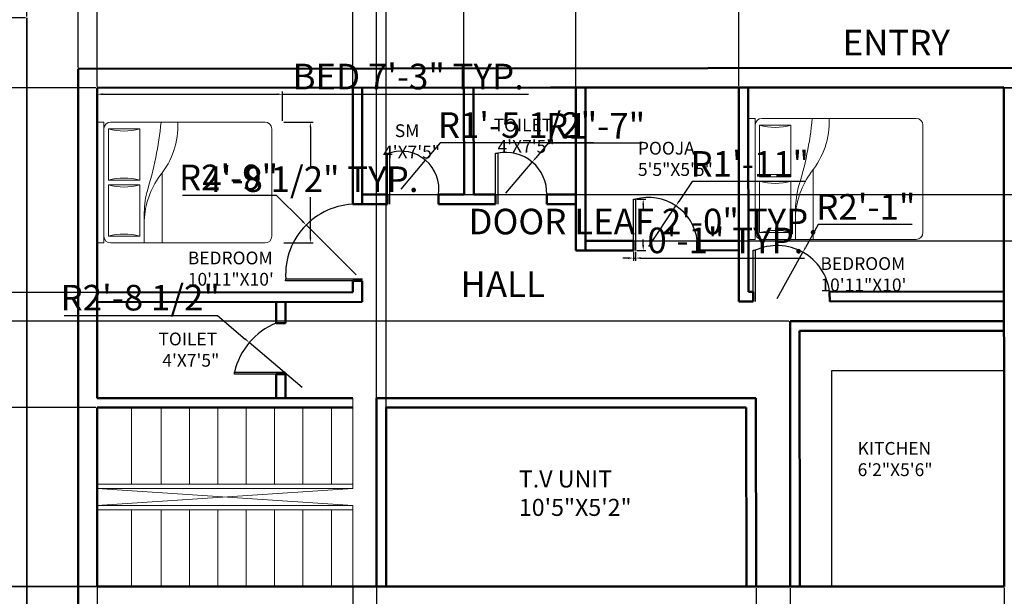
# Model space of a CAD drawing. Units: inches. Extents: x 5307 to 6359, y 4763 to 5474.
# Tile 3 of 5: x 5543 to 6006, y 4966 to 5237. Entities that reach past the tile are written whole.
import ezdxf
from ezdxf.enums import TextEntityAlignment as Align

# ---------------------------------------------------------------- set-up
doc = ezdxf.new("R2010")
doc.units = ezdxf.units.IN
for name, color, linetype, lineweight in [('A-ANNO-DIMS', 2, 'Continuous', 18), ('A-ANNO-TEXT', 7, 'Continuous', 18), ('A-AREA-IDEN', 7, 'Continuous', 18), ('A-DOOR', 4, 'Continuous', 25), ('A-FLOR-FIXT', 9, 'Continuous', 25), ('A-FLOR-STRS', 3, 'Continuous', 18), ('A-WALL', 7, 'Continuous', 50), ('C-PROP', 7, 'Continuous', 35), ('FUR', 42, 'Continuous', 18)]:
    doc.layers.add(name, color=color, linetype=linetype, lineweight=lineweight)
doc.styles.add('ATT', font='romans.shx')
doc.styles.get("Standard").update_dxf_attribs({"font": 'arial.ttf'})
doc.dimstyles.new('ISO-25', dxfattribs={"dimtxt": 12, "dimasz": 2.5, "dimexe": 1.25, "dimexo": 0.625, "dimtad": 1, "dimtih": 1, "dimtoh": 1, "dimlunit": 4, "dimtxsty": 'Standard', "dimcen": 2.5, "dimadec": 0, "dimazin": 0, "dimtfac": 1, "dimtmove": 0, "dimatfit": 3, "dimfxl": 1, "dimarcsym": 0})

# ---------------------------------------------------------------- blocks, each defined once
blk = doc.blocks.new('*D3')
at = {"layer": 'A-ANNO-DIMS', "color": 0, "lineweight": -2, "transparency": 16777216}
for p, q in [((5545.97, 5237.78), (5511.45, 5237.78)), ((5512.7, 5235.28), (5512.7, 5094.54)), ((5512.7, 4940.28), (5512.7, 5081.03)), ((5545.97, 4937.78), (5511.45, 4937.78))]:
    blk.add_line(p, q, dxfattribs=at)
at = {"layer": 'A-ANNO-DIMS', "color": 0, "transparency": 16777216}
for points in [[(5512.28, 5235.28), (5513.12, 5235.28), (5512.7, 5237.78)], [(5512.28, 4940.28), (5513.12, 4940.28), (5512.7, 4937.78)]]:
    blk.add_solid(points, dxfattribs=at)
at = {"layer": 'Defpoints', "color": 0, "transparency": 16777216}
for p in [(5546.59, 5237.78), (5512.7, 4937.78), (5546.59, 4937.78)]:
    blk.add_point(p, dxfattribs=at)
at = {"layer": 'A-ANNO-DIMS', "color": 0, "transparency": 16777216, "insert": (5512.7, 5087.78), "char_height": 12, "attachment_point": 5}
blk.add_mtext("25'", dxfattribs=at)
blk = doc.blocks.new('12PBED03')
at = {"color": 0, "linetype": 'ByBlock'}
for p, q in [((3, 54), (0, 54)), ((0, 0), (0, 54)), ((3, 0), (3, 54)), ((6, 54), (75, 54)), ((21, 41.758136), (21, 54)), ((29, 23), (29, 54)), ((19, 51), (5, 51)), ((5, 51), (5, 28)), ((19, 28), (19, 51)), ((78, 51), (78, 3)), ((5, 28), (19, 28)), ((5, 26), (5, 3)), ((19, 26), (5, 26)), ((19, 3), (19, 26)), ((3, 0), (0, 0)), ((5, 3), (19, 3)), ((75, 0), (6, 0))]:
    blk.add_line(p, q, dxfattribs=at)
for centre, radius, start, end in [((6, 51), 3, 90, 180), ((75, 51), 3, 0, 90), ((12, 75), 25, 253.739795, 286.260205), ((69.004289, 41.742518), 48.004291, 179.981359, 192.466744), ((57.725806, 45.629032), 36.761918, 182.539782, 216.040311), ((-120.191801, -13.95004), 149.36804, 5.357156, 17.666547), ((12, 4), 25, 73.739795, 106.260205), ((12, 50), 25, 253.739795, 286.260205), ((0.75, 1.5), 35.338541, 357.56726, 39.546081), ((6, 3), 3, 180, 270), ((12, -21), 25, 73.739795, 106.260205), ((75, 3), 3, 270, 0)]:
    blk.add_arc(centre, radius, start, end, dxfattribs=at)
at = {"color": 0, "linetype": 'ByBlock', "style": 'ATT'}
for tag, flags, p in [('ITEM', 3, (50, 33)), ('ROOM_NUMBER', 1, (50, 18.5))]:
    blk.add_attdef(tag, text='', height=6, dxfattribs=dict(at, flags=flags)).set_placement(p, align=Align.CENTER)
blk = doc.blocks.new('DOOR-LEAF-24IN')
for p, q in [((0, 0), (0, 24)), ((0, 24), (1, 24)), ((1, 24), (1, 0))]:
    blk.add_line(p, q)
blk = doc.blocks.new('*D8')
at = {"layer": 'A-ANNO-DIMS', "color": 0, "lineweight": -2, "transparency": 16777216}
for p, q in [((5833.01, 5152.56), (5837.24, 5152.56)), ((5835.99, 5150.06), (5835.99, 5147.39)), ((5835.99, 5131.06), (5835.99, 5133.73)), ((5833.01, 5128.56), (5837.24, 5128.56))]:
    blk.add_line(p, q, dxfattribs=at)
at = {"layer": 'A-ANNO-DIMS', "color": 0, "transparency": 16777216}
for points in [[(5835.57, 5150.06), (5836.4, 5150.06), (5835.99, 5152.56)], [(5835.57, 5131.06), (5836.4, 5131.06), (5835.99, 5128.56)]]:
    blk.add_solid(points, dxfattribs=at)
at = {"layer": 'Defpoints', "color": 0, "transparency": 16777216}
for p in [(5832.39, 5152.56), (5835.99, 5152.56), (5832.39, 5128.56)]:
    blk.add_point(p, dxfattribs=at)
at = {"layer": 'A-ANNO-DIMS', "color": 0, "transparency": 16777216, "insert": (5835.99, 5140.56), "char_height": 12, "attachment_point": 5}
blk.add_mtext('DOOR LEAF 2\'-0" TYP.', dxfattribs=at)
blk = doc.blocks.new('*D9')
at = {"layer": 'A-ANNO-DIMS', "color": 0, "lineweight": -2, "transparency": 16777216}
for p, q in [((5831.39, 5127.94), (5831.39, 5123.71)), ((5832.39, 5127.94), (5832.39, 5123.71)), ((5828.89, 5124.96), (5826.39, 5124.96)), ((5831.39, 5124.96), (5832.39, 5124.96)), ((5834.89, 5124.96), (5911.78, 5124.96))]:
    blk.add_line(p, q, dxfattribs=at)
at = {"layer": 'A-ANNO-DIMS', "color": 0, "transparency": 16777216}
for points in [[(5828.89, 5125.38), (5828.89, 5124.54), (5831.39, 5124.96)], [(5834.89, 5125.38), (5834.89, 5124.54), (5832.39, 5124.96)]]:
    blk.add_solid(points, dxfattribs=at)
at = {"layer": 'Defpoints', "color": 0, "transparency": 16777216}
for p in [(5831.39, 5128.56), (5832.39, 5128.56), (5832.39, 5124.96)]:
    blk.add_point(p, dxfattribs=at)
at = {"layer": 'A-ANNO-DIMS', "color": 0, "transparency": 16777216, "insert": (5874.59, 5131.71), "char_height": 12, "attachment_point": 5}
blk.add_mtext('0\'-1" TYP.', dxfattribs=at)
blk = doc.blocks.new('*D10')
at = {"layer": 'A-ANNO-DIMS', "color": 0, "lineweight": -2, "transparency": 16777216}
for p, q in [((5579.59, 5189.42), (5579.59, 5203.11)), ((5582.09, 5201.86), (5664.17, 5201.86)), ((5666.67, 5189.42), (5666.67, 5203.11)), ((5666.67, 5201.86), (5782.16, 5201.86))]:
    blk.add_line(p, q, dxfattribs=at)
at = {"layer": 'A-ANNO-DIMS', "color": 0, "transparency": 16777216}
for points in [[(5582.09, 5202.27), (5582.09, 5201.44), (5579.59, 5201.86)], [(5664.17, 5202.27), (5664.17, 5201.44), (5666.67, 5201.86)]]:
    blk.add_solid(points, dxfattribs=at)
at = {"layer": 'Defpoints', "color": 0, "transparency": 16777216}
for p in [(5666.67, 5201.86), (5579.59, 5188.79), (5666.67, 5188.79)]:
    blk.add_point(p, dxfattribs=at)
at = {"layer": 'A-ANNO-DIMS', "color": 0, "transparency": 16777216, "insert": (5725.66, 5208.61), "char_height": 12, "attachment_point": 5}
blk.add_mtext('BED 7\'-3" TYP.', dxfattribs=at)
blk = doc.blocks.new('*D11')
at = {"layer": 'A-ANNO-DIMS', "color": 0, "lineweight": -2, "transparency": 16777216}
for p, q in [((5667.29, 5188.79), (5680.98, 5188.79)), ((5679.73, 5186.29), (5679.73, 5167.25)), ((5679.73, 5134.55), (5679.73, 5153.59)), ((5667.29, 5132.05), (5680.98, 5132.05))]:
    blk.add_line(p, q, dxfattribs=at)
at = {"layer": 'A-ANNO-DIMS', "color": 0, "transparency": 16777216}
for points in [[(5679.31, 5186.29), (5680.14, 5186.29), (5679.73, 5188.79)], [(5679.31, 5134.55), (5680.14, 5134.55), (5679.73, 5132.05)]]:
    blk.add_solid(points, dxfattribs=at)
at = {"layer": 'Defpoints', "color": 0, "transparency": 16777216}
for p in [(5666.67, 5188.79), (5666.67, 5132.05), (5679.73, 5132.05)]:
    blk.add_point(p, dxfattribs=at)
at = {"layer": 'A-ANNO-DIMS', "color": 0, "transparency": 16777216, "insert": (5679.73, 5160.42), "char_height": 12, "attachment_point": 5}
blk.add_mtext('4\'-8 1/2" TYP.', dxfattribs=at)
blk = doc.blocks.new('*D13')
at = {"layer": 'A-ANNO-DIMS', "color": 0, "lineweight": -2, "transparency": 16777216}
for p, q in [((6038.88, 5405.78), (6325.25, 5405.78)), ((6324, 5403.28), (6324, 5118.54)), ((6324, 4820.28), (6324, 5105.03)), ((5547.22, 4817.78), (6325.25, 4817.78))]:
    blk.add_line(p, q, dxfattribs=at)
at = {"layer": 'A-ANNO-DIMS', "color": 0, "transparency": 16777216}
for points in [[(6323.58, 5403.28), (6324.41, 5403.28), (6324, 5405.78)], [(6323.58, 4820.28), (6324.41, 4820.28), (6324, 4817.78)]]:
    blk.add_solid(points, dxfattribs=at)
at = {"layer": 'Defpoints', "color": 0, "transparency": 16777216}
for p in [(6038.25, 5405.78), (6324, 5405.78), (5546.59, 4817.78)]:
    blk.add_point(p, dxfattribs=at)
at = {"layer": 'A-ANNO-DIMS', "color": 0, "transparency": 16777216, "insert": (6324, 5111.78), "char_height": 12, "attachment_point": 5}
blk.add_mtext('49\'-0"', dxfattribs=at)
blk = doc.blocks.new('*D14')
at = {"layer": 'A-ANNO-DIMS', "color": 0, "lineweight": -2, "transparency": 16777216}
for p, q in [((5546.59, 5238.41), (5546.59, 5450.78)), ((5549.09, 5449.53), (5568.09, 5449.53)), ((5570.59, 5214.43), (5570.59, 5450.78)), ((5570.59, 5449.53), (5606.45, 5449.53))]:
    blk.add_line(p, q, dxfattribs=at)
at = {"layer": 'A-ANNO-DIMS', "color": 0, "transparency": 16777216}
for points in [[(5549.09, 5449.95), (5549.09, 5449.12), (5546.59, 5449.53)], [(5568.09, 5449.95), (5568.09, 5449.12), (5570.59, 5449.53)]]:
    blk.add_solid(points, dxfattribs=at)
at = {"layer": 'Defpoints', "color": 0, "transparency": 16777216}
for p in [(5570.59, 5449.53), (5546.59, 5237.78), (5570.59, 5213.81)]:
    blk.add_point(p, dxfattribs=at)
at = {"layer": 'A-ANNO-DIMS', "color": 0, "transparency": 16777216, "insert": (5589.77, 5456.29), "char_height": 12, "attachment_point": 5}
blk.add_mtext('2\'-0"', dxfattribs=at)
blk = doc.blocks.new('*D19')
at = {"layer": 'A-ANNO-DIMS', "color": 0, "lineweight": -2, "transparency": 16777216}
for p, q in [((5570.59, 5214.43), (5570.59, 5450.78)), ((5573.09, 5449.53), (5577.09, 5449.53)), ((5579.59, 5205.44), (5579.59, 5450.78)), ((5579.59, 5449.53), (5615.24, 5449.53))]:
    blk.add_line(p, q, dxfattribs=at)
at = {"layer": 'A-ANNO-DIMS', "color": 0, "transparency": 16777216}
for points in [[(5573.09, 5449.95), (5573.09, 5449.12), (5570.59, 5449.53)], [(5577.09, 5449.95), (5577.09, 5449.12), (5579.59, 5449.53)]]:
    blk.add_solid(points, dxfattribs=at)
at = {"layer": 'Defpoints', "color": 0, "transparency": 16777216}
for p in [(5579.59, 5449.53), (5570.59, 5213.81), (5579.59, 5204.82)]:
    blk.add_point(p, dxfattribs=at)
at = {"layer": 'A-ANNO-DIMS', "color": 0, "transparency": 16777216, "insert": (5598.67, 5456.29), "char_height": 12, "attachment_point": 5}
blk.add_mtext('0\'-9"', dxfattribs=at)
blk = doc.blocks.new('*D20')
at = {"layer": 'A-ANNO-DIMS', "color": 0, "lineweight": -2, "transparency": 16777216}
for p, q in [((5579.59, 5205.44), (5579.59, 5450.78)), ((5582.09, 5449.53), (5697.09, 5449.53)), ((5699.59, 5205.56), (5699.59, 5450.78))]:
    blk.add_line(p, q, dxfattribs=at)
at = {"layer": 'A-ANNO-DIMS', "color": 0, "transparency": 16777216}
for points in [[(5582.09, 5449.95), (5582.09, 5449.12), (5579.59, 5449.53)], [(5697.09, 5449.95), (5697.09, 5449.12), (5699.59, 5449.53)]]:
    blk.add_solid(points, dxfattribs=at)
at = {"layer": 'Defpoints', "color": 0, "transparency": 16777216}
for p in [(5699.59, 5449.53), (5579.59, 5204.82), (5699.59, 5204.93)]:
    blk.add_point(p, dxfattribs=at)
at = {"layer": 'A-ANNO-DIMS', "color": 0, "transparency": 16777216, "insert": (5639.59, 5456.29), "char_height": 12, "attachment_point": 5}
blk.add_mtext('10\'-0"', dxfattribs=at)
blk = doc.blocks.new('*D21')
at = {"layer": 'A-ANNO-DIMS', "color": 0, "lineweight": -2, "transparency": 16777216}
for p, q in [((5699.59, 5205.56), (5699.59, 5450.78)), ((5702.09, 5449.53), (5749.33, 5449.53)), ((5751.83, 5205.61), (5751.83, 5450.78))]:
    blk.add_line(p, q, dxfattribs=at)
at = {"layer": 'A-ANNO-DIMS', "color": 0, "transparency": 16777216}
for points in [[(5702.09, 5449.95), (5702.09, 5449.12), (5699.59, 5449.53)], [(5749.33, 5449.95), (5749.33, 5449.12), (5751.83, 5449.53)]]:
    blk.add_solid(points, dxfattribs=at)
at = {"layer": 'Defpoints', "color": 0, "transparency": 16777216}
for p in [(5751.83, 5449.53), (5699.59, 5204.93), (5751.83, 5204.98)]:
    blk.add_point(p, dxfattribs=at)
at = {"layer": 'A-ANNO-DIMS', "color": 0, "transparency": 16777216, "insert": (5725.71, 5456.16), "char_height": 12, "attachment_point": 5}
blk.add_mtext('4\'-4"', dxfattribs=at)
blk = doc.blocks.new('*D22')
at = {"layer": 'A-ANNO-DIMS', "color": 0, "lineweight": -2, "transparency": 16777216}
for p, q in [((5751.83, 5205.61), (5751.83, 5450.78)), ((5754.33, 5449.53), (5801.83, 5449.53)), ((5804.33, 5205.66), (5804.33, 5450.78)), ((5804.33, 5449.53), (5868.43, 5449.53))]:
    blk.add_line(p, q, dxfattribs=at)
at = {"layer": 'A-ANNO-DIMS', "color": 0, "transparency": 16777216}
for points in [[(5754.33, 5449.95), (5754.33, 5449.12), (5751.83, 5449.53)], [(5801.83, 5449.95), (5801.83, 5449.12), (5804.33, 5449.53)]]:
    blk.add_solid(points, dxfattribs=at)
at = {"layer": 'Defpoints', "color": 0, "transparency": 16777216}
for p in [(5804.33, 5449.53), (5751.83, 5204.98), (5804.33, 5205.03)]:
    blk.add_point(p, dxfattribs=at)
at = {"layer": 'A-ANNO-DIMS', "color": 0, "transparency": 16777216, "insert": (5837.63, 5456.36), "char_height": 12, "attachment_point": 5}
blk.add_mtext('4\'-4 1/2"', dxfattribs=at)
blk = doc.blocks.new('*D23')
at = {"layer": 'A-ANNO-DIMS', "color": 0, "lineweight": -2, "transparency": 16777216}
for p, q in [((5804.33, 5205.66), (5804.33, 5450.78)), ((5806.83, 5449.53), (5878.33, 5449.53)), ((5880.83, 5205.73), (5880.83, 5450.78))]:
    blk.add_line(p, q, dxfattribs=at)
at = {"layer": 'A-ANNO-DIMS', "color": 0, "transparency": 16777216}
for points in [[(5806.83, 5449.95), (5806.83, 5449.12), (5804.33, 5449.53)], [(5878.33, 5449.95), (5878.33, 5449.12), (5880.83, 5449.53)]]:
    blk.add_solid(points, dxfattribs=at)
at = {"layer": 'Defpoints', "color": 0, "transparency": 16777216}
for p in [(5880.83, 5449.53), (5804.33, 5205.03), (5880.83, 5205.11)]:
    blk.add_point(p, dxfattribs=at)
at = {"layer": 'A-ANNO-DIMS', "color": 0, "transparency": 16777216, "insert": (5842.58, 5456.36), "char_height": 12, "attachment_point": 5}
blk.add_mtext('6\'-4 1/2"', dxfattribs=at)
blk = doc.blocks.new('*D24')
at = {"layer": 'A-ANNO-DIMS', "color": 0, "lineweight": -2, "transparency": 16777216}
for p, q in [((5579.59, 4970.16), (5579.59, 4772.78)), ((5699.59, 4970.16), (5699.59, 4772.78)), ((5582.09, 4774.03), (5697.09, 4774.03))]:
    blk.add_line(p, q, dxfattribs=at)
at = {"layer": 'A-ANNO-DIMS', "color": 0, "transparency": 16777216}
for points in [[(5582.09, 4774.45), (5582.09, 4773.62), (5579.59, 4774.03)], [(5697.09, 4774.45), (5697.09, 4773.62), (5699.59, 4774.03)]]:
    blk.add_solid(points, dxfattribs=at)
at = {"layer": 'Defpoints', "color": 0, "transparency": 16777216}
for p in [(5579.59, 4970.78), (5699.59, 4970.78), (5699.59, 4774.03)]:
    blk.add_point(p, dxfattribs=at)
at = {"layer": 'A-ANNO-DIMS', "color": 0, "transparency": 16777216, "insert": (5639.59, 4780.79), "char_height": 12, "attachment_point": 5}
blk.add_mtext('10\'-0"', dxfattribs=at)
blk = doc.blocks.new('*D25')
at = {"layer": 'A-ANNO-DIMS', "color": 0, "lineweight": -2, "transparency": 16777216}
for p, q in [((5710.76, 4970.16), (5710.76, 4772.78)), ((5889, 4970.05), (5889, 4772.78)), ((5713.26, 4774.03), (5886.5, 4774.03))]:
    blk.add_line(p, q, dxfattribs=at)
at = {"layer": 'A-ANNO-DIMS', "color": 0, "transparency": 16777216}
for points in [[(5713.26, 4774.45), (5713.26, 4773.62), (5710.76, 4774.03)], [(5886.5, 4774.45), (5886.5, 4773.62), (5889, 4774.03)]]:
    blk.add_solid(points, dxfattribs=at)
at = {"layer": 'Defpoints', "color": 0, "transparency": 16777216}
for p in [(5710.76, 4970.78), (5889, 4970.67), (5889, 4774.03)]:
    blk.add_point(p, dxfattribs=at)
at = {"layer": 'A-ANNO-DIMS', "color": 0, "transparency": 16777216, "insert": (5799.88, 4780.79), "char_height": 12, "attachment_point": 5}
blk.add_mtext('14\'-10"', dxfattribs=at)
blk = doc.blocks.new('*D26')
at = {"layer": 'A-ANNO-DIMS', "color": 0, "lineweight": -2, "transparency": 16777216}
for p, q in [((5905.06, 4970.06), (5905.06, 4772.78)), ((6005.56, 4970.16), (6005.56, 4772.78)), ((5907.56, 4774.03), (6003.06, 4774.03))]:
    blk.add_line(p, q, dxfattribs=at)
at = {"layer": 'A-ANNO-DIMS', "color": 0, "transparency": 16777216}
for points in [[(5907.56, 4774.45), (5907.56, 4773.62), (5905.06, 4774.03)], [(6003.06, 4774.45), (6003.06, 4773.62), (6005.56, 4774.03)]]:
    blk.add_solid(points, dxfattribs=at)
at = {"layer": 'Defpoints', "color": 0, "transparency": 16777216}
for p in [(5905.06, 4970.69), (6005.56, 4970.78), (6005.56, 4774.03)]:
    blk.add_point(p, dxfattribs=at)
at = {"layer": 'A-ANNO-DIMS', "color": 0, "transparency": 16777216, "insert": (5955.31, 4780.86), "char_height": 12, "attachment_point": 5}
blk.add_mtext('8\'-4 1/2"', dxfattribs=at)
blk = doc.blocks.new('*D27')
at = {"layer": 'A-ANNO-DIMS', "color": 0, "lineweight": -2, "transparency": 16777216}
for p, q in [((5578.97, 5054.78), (5381.59, 5054.78)), ((5382.84, 5052.28), (5382.84, 5019.54)), ((5382.84, 4973.28), (5382.84, 5006.03)), ((5578.97, 4970.78), (5381.59, 4970.78))]:
    blk.add_line(p, q, dxfattribs=at)
at = {"layer": 'A-ANNO-DIMS', "color": 0, "transparency": 16777216}
for points in [[(5382.43, 5052.28), (5383.26, 5052.28), (5382.84, 5054.78)], [(5382.43, 4973.28), (5383.26, 4973.28), (5382.84, 4970.78)]]:
    blk.add_solid(points, dxfattribs=at)
at = {"layer": 'Defpoints', "color": 0, "transparency": 16777216}
for p in [(5382.84, 5054.78), (5579.59, 5054.78), (5579.59, 4970.78)]:
    blk.add_point(p, dxfattribs=at)
at = {"layer": 'A-ANNO-DIMS', "color": 0, "transparency": 16777216, "insert": (5382.84, 5012.78), "char_height": 12, "attachment_point": 5}
blk.add_mtext('7\'-0"', dxfattribs=at)
blk = doc.blocks.new('*D28')
at = {"layer": 'A-ANNO-DIMS', "color": 0, "lineweight": -2, "transparency": 16777216}
for p, q in [((5578.97, 5204.82), (5381.59, 5204.82)), ((5382.84, 5202.32), (5382.84, 5163.57)), ((5382.84, 5111.32), (5382.84, 5150.06)), ((5578.97, 5108.82), (5381.59, 5108.82))]:
    blk.add_line(p, q, dxfattribs=at)
at = {"layer": 'A-ANNO-DIMS', "color": 0, "transparency": 16777216}
for points in [[(5382.43, 5202.32), (5383.26, 5202.32), (5382.84, 5204.82)], [(5382.43, 5111.32), (5383.26, 5111.32), (5382.84, 5108.82)]]:
    blk.add_solid(points, dxfattribs=at)
at = {"layer": 'Defpoints', "color": 0, "transparency": 16777216}
for p in [(5382.84, 5204.82), (5579.59, 5204.82), (5579.59, 5108.82)]:
    blk.add_point(p, dxfattribs=at)
at = {"layer": 'A-ANNO-DIMS', "color": 0, "transparency": 16777216, "insert": (5382.84, 5156.82), "char_height": 12, "attachment_point": 5}
blk.add_mtext('8\'-0"', dxfattribs=at)
blk = doc.blocks.new('*D29')
at = {"layer": 'A-ANNO-DIMS', "color": 0, "lineweight": -2, "transparency": 16777216}
for p, q in [((5904.31, 5095.28), (5381.59, 5095.28)), ((5382.84, 5092.78), (5382.84, 5039.81)), ((5382.84, 4973.19), (5382.84, 5026.16)), ((5904.44, 4970.69), (5381.59, 4970.69))]:
    blk.add_line(p, q, dxfattribs=at)
at = {"layer": 'A-ANNO-DIMS', "color": 0, "transparency": 16777216}
for points in [[(5382.43, 5092.78), (5383.26, 5092.78), (5382.84, 5095.28)], [(5382.43, 4973.19), (5383.26, 4973.19), (5382.84, 4970.69)]]:
    blk.add_solid(points, dxfattribs=at)
at = {"layer": 'Defpoints', "color": 0, "transparency": 16777216}
for p in [(5382.84, 5095.28), (5904.94, 5095.28), (5905.06, 4970.69)]:
    blk.add_point(p, dxfattribs=at)
at = {"layer": 'A-ANNO-DIMS', "color": 0, "transparency": 16777216, "insert": (5382.84, 5032.99), "char_height": 12, "attachment_point": 5}
blk.add_mtext('10\'-4 1/2"', dxfattribs=at)
blk = doc.blocks.new('*D30')
at = {"layer": 'A-ANNO-DIMS', "color": 0, "lineweight": -2, "transparency": 16777216}
for p, q in [((5708.26, 5449.53), (5705.76, 5449.53)), ((5710.76, 4971.41), (5710.76, 5450.78)), ((5710.76, 5449.53), (5715.26, 5449.53)), ((5715.26, 4971.41), (5715.26, 5450.78)), ((5717.76, 5449.53), (5781.37, 5449.53))]:
    blk.add_line(p, q, dxfattribs=at)
at = {"layer": 'A-ANNO-DIMS', "color": 0, "transparency": 16777216}
for points in [[(5708.26, 5449.95), (5708.26, 5449.12), (5710.76, 5449.53)], [(5717.76, 5449.95), (5717.76, 5449.12), (5715.26, 5449.53)]]:
    blk.add_solid(points, dxfattribs=at)
at = {"layer": 'Defpoints', "color": 0, "transparency": 16777216}
for p in [(5715.26, 5449.53), (5710.76, 4970.78), (5715.26, 4970.78)]:
    blk.add_point(p, dxfattribs=at)
at = {"layer": 'A-ANNO-DIMS', "color": 0, "transparency": 16777216, "insert": (5750.81, 5456.36), "char_height": 12, "attachment_point": 5}
blk.add_mtext('0\'-4 1/2"', dxfattribs=at)
blk = doc.blocks.new('*D31')
at = {"layer": 'A-ANNO-DIMS', "color": 0, "lineweight": -2, "transparency": 16777216}
for p, q in [((5704.72, 5204.94), (6325.25, 5204.94)), ((6324, 5202.44), (6324, 5186.48)), ((6324, 5157.23), (6324, 5173.19)), ((5704.72, 5154.73), (6325.25, 5154.73))]:
    blk.add_line(p, q, dxfattribs=at)
at = {"layer": 'A-ANNO-DIMS', "color": 0, "transparency": 16777216}
for points in [[(6323.58, 5202.44), (6324.41, 5202.44), (6324, 5204.94)], [(6323.58, 5157.23), (6324.41, 5157.23), (6324, 5154.73)]]:
    blk.add_solid(points, dxfattribs=at)
at = {"layer": 'Defpoints', "color": 0, "transparency": 16777216}
for p in [(5704.09, 5204.94), (6324, 5204.94), (5704.09, 5154.73)]:
    blk.add_point(p, dxfattribs=at)
at = {"layer": 'A-ANNO-DIMS', "color": 0, "transparency": 16777216, "insert": (6324, 5179.83), "char_height": 12, "attachment_point": 5}
blk.add_mtext('4\'-2"', dxfattribs=at)
blk = doc.blocks.new('*D32')
at = {"layer": 'A-ANNO-DIMS', "color": 0, "lineweight": -2, "transparency": 16777216}
for p, q in [((5809.46, 5205.04), (6325.25, 5205.04)), ((6324, 5202.54), (6324, 5175.79)), ((6324, 5135.54), (6324, 5162.29)), ((5809.53, 5133.04), (6325.25, 5133.04))]:
    blk.add_line(p, q, dxfattribs=at)
at = {"layer": 'A-ANNO-DIMS', "color": 0, "transparency": 16777216}
for points in [[(6323.58, 5202.54), (6324.41, 5202.54), (6324, 5205.04)], [(6323.58, 5135.54), (6324.41, 5135.54), (6324, 5133.04)]]:
    blk.add_solid(points, dxfattribs=at)
at = {"layer": 'Defpoints', "color": 0, "transparency": 16777216}
for p in [(5808.83, 5205.04), (6324, 5205.04), (5808.9, 5133.04)]:
    blk.add_point(p, dxfattribs=at)
at = {"layer": 'A-ANNO-DIMS', "color": 0, "transparency": 16777216, "insert": (6324, 5169.04), "char_height": 12, "attachment_point": 5}
blk.add_mtext('6\'-0"', dxfattribs=at)
blk = doc.blocks.new('*D35')
at = {"layer": 'A-ANNO-DIMS', "color": 0, "lineweight": -2, "transparency": 16777216}
for p, q in [((5619.59, 5154.53), (5663.6, 5154.53)), ((5663.6, 5154.53), (5675.95, 5142.25)), ((5701.26, 5117.08), (5677.72, 5140.49))]:
    blk.add_line(p, q, dxfattribs=at)
at = {"layer": 'A-ANNO-DIMS', "color": 0, "transparency": 16777216}
blk.add_solid([(5676.24, 5142.55), (5675.65, 5141.95), (5677.72, 5140.49)], dxfattribs=at)
at = {"layer": 'Defpoints', "color": 0, "transparency": 16777216}
for p in [(5677.72, 5140.49), (5701.26, 5117.08)]:
    blk.add_point(p, dxfattribs=at)
at = {"layer": 'A-ANNO-DIMS', "color": 0, "transparency": 16777216, "insert": (5641.28, 5161.28), "char_height": 12, "attachment_point": 5}
blk.add_mtext('R2\'-9"', dxfattribs=at)
blk = doc.blocks.new('*D36')
at = {"layer": 'A-ANNO-DIMS', "color": 0, "lineweight": -2, "transparency": 16777216}
for p, q in [((5564.14, 5098), (5636.11, 5098)), ((5636.11, 5098), (5649.11, 5086.98)), ((5675.87, 5064.29), (5651.02, 5085.36))]:
    blk.add_line(p, q, dxfattribs=at)
at = {"layer": 'A-ANNO-DIMS', "color": 0, "transparency": 16777216}
blk.add_solid([(5649.38, 5087.29), (5648.85, 5086.66), (5651.02, 5085.36)], dxfattribs=at)
at = {"layer": 'Defpoints', "color": 0, "transparency": 16777216}
for p in [(5651.02, 5085.36), (5675.87, 5064.29)]:
    blk.add_point(p, dxfattribs=at)
at = {"layer": 'A-ANNO-DIMS', "color": 0, "transparency": 16777216, "insert": (5599.81, 5104.83), "char_height": 12, "attachment_point": 5}
blk.add_mtext('R2\'-8 1/2"', dxfattribs=at)
blk = doc.blocks.new('*D37')
at = {"layer": 'A-ANNO-DIMS', "color": 0, "lineweight": -2, "transparency": 16777216}
for p, q in [((5918.23, 5140.77), (5912.18, 5129.89)), ((5962.24, 5140.77), (5918.23, 5140.77)), ((5898.85, 5105.95), (5910.97, 5127.71))]:
    blk.add_line(p, q, dxfattribs=at)
at = {"layer": 'A-ANNO-DIMS', "color": 0, "transparency": 16777216}
blk.add_solid([(5911.82, 5130.1), (5912.54, 5129.69), (5910.97, 5127.71)], dxfattribs=at)
at = {"layer": 'Defpoints', "color": 0, "transparency": 16777216}
for p in [(5910.97, 5127.71), (5898.85, 5105.95)]:
    blk.add_point(p, dxfattribs=at)
at = {"layer": 'A-ANNO-DIMS', "color": 0, "transparency": 16777216, "insert": (5940.55, 5147.42), "char_height": 12, "attachment_point": 5}
blk.add_mtext('R2\'-1"', dxfattribs=at)
blk = doc.blocks.new('*D38')
at = {"layer": 'A-ANNO-DIMS', "color": 0, "lineweight": -2, "transparency": 16777216}
for p, q in [((5859.06, 5160.95), (5852.76, 5151.58)), ((5912.39, 5160.95), (5859.06, 5160.95)), ((5838.56, 5130.42), (5851.37, 5149.5))]:
    blk.add_line(p, q, dxfattribs=at)
at = {"layer": 'A-ANNO-DIMS', "color": 0, "transparency": 16777216}
blk.add_solid([(5852.42, 5151.81), (5853.11, 5151.34), (5851.37, 5149.5)], dxfattribs=at)
at = {"layer": 'Defpoints', "color": 0, "transparency": 16777216}
for p in [(5851.37, 5149.5), (5838.56, 5130.42)]:
    blk.add_point(p, dxfattribs=at)
at = {"layer": 'A-ANNO-DIMS', "color": 0, "transparency": 16777216, "insert": (5886.03, 5167.6), "char_height": 12, "attachment_point": 5}
blk.add_mtext('R1\'-11"', dxfattribs=at)
blk = doc.blocks.new('*D39')
at = {"layer": 'A-ANNO-DIMS', "color": 0, "lineweight": -2, "transparency": 16777216}
for p, q in [((5791.33, 5178.82), (5785.53, 5171.95)), ((5835.34, 5178.82), (5791.33, 5178.82)), ((5771.55, 5155.4), (5783.91, 5170.04))]:
    blk.add_line(p, q, dxfattribs=at)
at = {"layer": 'A-ANNO-DIMS', "color": 0, "transparency": 16777216}
blk.add_solid([(5785.21, 5172.21), (5785.84, 5171.68), (5783.91, 5170.04)], dxfattribs=at)
at = {"layer": 'Defpoints', "color": 0, "transparency": 16777216}
for p in [(5783.91, 5170.04), (5771.55, 5155.4)]:
    blk.add_point(p, dxfattribs=at)
at = {"layer": 'A-ANNO-DIMS', "color": 0, "transparency": 16777216, "insert": (5813.64, 5185.46), "char_height": 12, "attachment_point": 5}
blk.add_mtext('R1\'-7"', dxfattribs=at)
blk = doc.blocks.new('*D40')
at = {"layer": 'A-ANNO-DIMS', "color": 0, "lineweight": -2, "transparency": 16777216}
for p, q in [((5740.66, 5179), (5735.4, 5172.79)), ((5812.63, 5179), (5740.66, 5179)), ((5722.31, 5157.36), (5733.78, 5170.89))]:
    blk.add_line(p, q, dxfattribs=at)
at = {"layer": 'A-ANNO-DIMS', "color": 0, "transparency": 16777216}
blk.add_solid([(5735.08, 5173.06), (5735.72, 5172.52), (5733.78, 5170.89)], dxfattribs=at)
at = {"layer": 'Defpoints', "color": 0, "transparency": 16777216}
for p in [(5733.78, 5170.89), (5722.31, 5157.36)]:
    blk.add_point(p, dxfattribs=at)
at = {"layer": 'A-ANNO-DIMS', "color": 0, "transparency": 16777216, "insert": (5776.96, 5185.83), "char_height": 12, "attachment_point": 5}
blk.add_mtext('R1\'-5 1/2"', dxfattribs=at)

msp = doc.modelspace()

# ---------------------------------------------------------------- linework, layer by layer
at = {"layer": 'A-DOOR'}
for p, q in [((5887.558, 5128.615), (5888.558, 5128.624)), ((5887.558, 5104.615), (5887.558, 5128.615)), ((5888.558, 5128.624), (5888.558, 5104.624)), ((5668.092, 5114.233), (5668.113, 5115.233)), ((5704.092, 5114.233), (5668.092, 5114.233)), ((5668.113, 5115.233), (5704.113, 5115.258))]:
    msp.add_line(p, q, dxfattribs=at)
for centre, radius, start, end in [((5722.312, 5157.356), 17.737, 351.4949, 107.9208), ((5771.552, 5155.403), 19.154, 358.00742, 101.6178), ((5838.558, 5130.423), 22.981, 6.66301, 105.57332), ((5701.257, 5117.08), 33.195, 87.1266, 183.18977), ((5898.855, 5105.946), 24.906, 7.39056, 114.41916), ((5675.874, 5064.289), 32.582, 112.14418, 167.27152)]:
    msp.add_arc(centre, radius, start, end, dxfattribs=at)
at = {"layer": 'A-FLOR-FIXT'}
for p, q in [((6005.462, 5071.994), (5924.438, 5071.994)), ((5924.438, 5071.994), (5924.438, 4970.784)), ((6005.462, 5071.994), (6005.462, 5071.994))]:
    msp.add_line(p, q, dxfattribs=at)
at = {"layer": 'A-FLOR-STRS'}
for p, q in [((5699.592, 5059.284), (5699.592, 5016.784)), ((5595.715, 5054.784), (5595.715, 5018.784)), ((5609.561, 5054.784), (5609.561, 5018.784)), ((5622.894, 5054.784), (5622.894, 5018.784)), ((5636.227, 5054.784), (5636.227, 5018.784)), ((5649.561, 5054.784), (5649.561, 5018.784)), ((5662.894, 5054.784), (5662.894, 5018.784)), ((5676.227, 5054.784), (5676.227, 5018.784)), ((5689.561, 5054.784), (5689.561, 5018.784)), ((5699.592, 5048.946), (5699.592, 5016.784)), ((5579.592, 5018.784), (5699.592, 5018.784)), ((5579.592, 5016.784), (5699.592, 5016.784)), ((5579.592, 5016.784), (5699.592, 5008.784)), ((5699.592, 5016.784), (5579.592, 5008.784)), ((5579.592, 5008.784), (5699.592, 5008.784)), ((5699.592, 5008.784), (5699.592, 4970.784)), ((5699.592, 5008.784), (5699.592, 4970.784)), ((5579.592, 5006.784), (5699.592, 5006.784)), ((5595.715, 5006.784), (5595.715, 4970.784)), ((5609.561, 5006.784), (5609.561, 4970.784)), ((5622.894, 5006.784), (5622.894, 4970.784)), ((5636.227, 5006.784), (5636.227, 4970.784)), ((5649.561, 5006.784), (5649.561, 4970.784)), ((5662.894, 5006.784), (5662.894, 4970.784)), ((5676.227, 5006.784), (5676.227, 4970.784)), ((5689.561, 5006.784), (5689.561, 4970.784))]:
    msp.add_line(p, q, dxfattribs=at)
at = {"layer": 'A-WALL'}
for p, q in [((5570.592, 5213.807), (6014.324, 5214.238)), ((5570.592, 5213.807), (5570.592, 4961.784)), ((5579.592, 5204.816), (6005.333, 5205.229)), ((5579.592, 5204.816), (5579.592, 5059.284)), ((5699.592, 5204.932), (5699.592, 5150.233)), ((5704.092, 5204.937), (5704.092, 5150.233)), ((5751.882, 5154.733), (5751.833, 5204.983)), ((5756.382, 5154.737), (5756.333, 5204.987)), ((5804.407, 5128.534), (5804.333, 5205.034)), ((5808.907, 5128.538), (5808.833, 5205.038)), ((5880.931, 5104.608), (5880.833, 5205.108)), ((5885.426, 5109.112), (5885.333, 5205.112)), ((6005.56, 4970.784), (6005.333, 5205.229)), ((5715.854, 5154.733), (5704.092, 5154.733)), ((5715.854, 5154.733), (5715.854, 5150.233)), ((5751.886, 5154.733), (5739.854, 5154.733)), ((5739.854, 5154.733), (5739.854, 5150.233)), ((5756.382, 5154.737), (5766.694, 5154.737)), ((5766.694, 5154.737), (5766.694, 5150.237)), ((5790.694, 5154.737), (5790.694, 5150.237)), ((5790.694, 5154.737), (5804.382, 5154.737)), ((5704.092, 5150.233), (5699.592, 5150.233)), ((5715.854, 5150.233), (5704.092, 5150.233)), ((5751.886, 5150.233), (5739.854, 5150.233)), ((5756.386, 5150.237), (5751.886, 5150.233)), ((5756.382, 5150.237), (5766.694, 5150.237)), ((5790.694, 5150.237), (5804.382, 5150.237)), ((5808.903, 5133.038), (5831.384, 5133.06)), ((5831.384, 5133.06), (5831.388, 5128.56)), ((5861.384, 5133.089), (5880.903, 5133.108)), ((5861.384, 5133.089), (5861.388, 5128.589)), ((5808.907, 5128.538), (5804.407, 5128.534)), ((5808.907, 5128.538), (5831.388, 5128.56)), ((5861.388, 5128.589), (5880.907, 5128.608)), ((5704.092, 5114.233), (5699.592, 5114.233)), ((5699.592, 5114.233), (5699.592, 5108.932)), ((5704.092, 5114.233), (5704.092, 5104.437)), ((5923.554, 5109.149), (6005.426, 5109.229)), ((5923.554, 5109.149), (5923.558, 5104.649)), ((5579.592, 5108.816), (5699.592, 5108.932)), ((5880.931, 5104.608), (5887.558, 5104.615)), ((5885.426, 5109.112), (5887.554, 5109.115)), ((5887.554, 5109.115), (5887.558, 5104.615)), ((5923.558, 5104.649), (6005.431, 5104.729)), ((5579.592, 5104.316), (5704.092, 5104.437)), ((5663.592, 5104.397), (5663.592, 5094.468)), ((5668.092, 5104.402), (5668.092, 5094.468)), ((5905.06, 4970.686), (5904.94, 5095.284)), ((5904.94, 5095.284), (6005.56, 5095.284)), ((5663.592, 5094.468), (5668.092, 5094.468)), ((5909.56, 4970.691), (5909.444, 5090.784)), ((5909.444, 5090.784), (6005.56, 5090.784)), ((5663.592, 5070.468), (5668.092, 5070.468)), ((5663.592, 5070.468), (5663.592, 5059.284)), ((5668.092, 5070.468), (5668.092, 5059.284)), ((5668.092, 5068.402), (5668.097, 5063.902)), ((5579.592, 5059.284), (5699.592, 5059.284)), ((5710.758, 5059.284), (5710.758, 4970.784)), ((5715.258, 5059.284), (5710.758, 5059.284)), ((5715.258, 5059.284), (5888.915, 5059.284)), ((5889.001, 4970.671), (5888.915, 5059.284)), ((6005.475, 5059.284), (6005.56, 5059.284)), ((5579.592, 5054.784), (5699.592, 5054.784)), ((5579.592, 5054.784), (5579.592, 4970.784)), ((5579.592, 5054.784), (5699.592, 5054.784)), ((5715.258, 5054.784), (5715.258, 4970.784)), ((5715.258, 5054.784), (5884.419, 5054.784)), ((5884.501, 4970.666), (5884.419, 5054.784)), ((6005.479, 5054.784), (6005.56, 5054.784)), ((5579.592, 4970.784), (5699.592, 4970.784)), ((5699.592, 4970.784), (6005.56, 4970.784))]:
    msp.add_line(p, q, dxfattribs=at)
at = {"layer": 'C-PROP'}
msp.add_line((5546.592, 5237.784), (5546.592, 4937.784), dxfattribs=at)

# ---------------------------------------------------------------- block references
at = {"layer": 'A-DOOR'}
for p in [(5715.854, 5150.233), (5766.694, 5150.237), (5831.388, 5128.56)]:
    msp.add_blockref('DOOR-LEAF-24IN', p, dxfattribs=at)
at = {"layer": 'A-DOOR', "rotation": 90.00000000000003}
msp.add_blockref('DOOR-LEAF-24IN', (5668.092, 5070.468), dxfattribs=at)
at = {"layer": 'FUR', "xscale": -1.050742393765131, "yscale": 1.050742393765131, "zscale": 1.050742393765131, "rotation": 180}
for p in [(5579.592, 5188.79), (5885.409, 5190.488)]:
    msp.add_blockref('12PBED03', p, dxfattribs=at)

# ---------------------------------------------------------------- texts
at = {"layer": 'A-ANNO-TEXT', "insert": (5929.636, 5232.102), "char_height": 12, "attachment_point": 1}
msp.add_mtext_dynamic_manual_height_columns('ENTRY', width=36.44889, gutter_width=12.5, heights=[0], dxfattribs=at)
at = {"layer": 'A-AREA-IDEN', "attachment_point": 1}
for s, width, insert, char_height in [('       SM\\P    4\'X7\'5"', 46.97276, (5706.522, 5187.748), 6), ('   TOILET\\P    4\'X7\'5"', 46.97276, (5760.255, 5190.374), 6), ('POOJA \\P5\'5"X5\'5"', 32.22485, (5833.51, 5179.529), 6), ('BEDROOM 10\'11"X10\'', 46.97276, (5622.148, 5128.023), 6), ('BEDROOM 10\'11"X10\'', 46.97276, (5919.219, 5125.38), 6), ('HALL', 63.71742, (5750.198, 5118.707), 12), ('   TOILET\\P    4\'X7\'5"', 46.97276, (5602.853, 5089.999), 6), ('KITCHEN\\P6\'2"X5\'6"', 53.87504, (5936.692, 5038.648), 6), ('T.V UNIT\\P10\'5"X5\'2"', 110.16563, (5777.591, 5025.291), 8)]:
    msp.add_mtext_dynamic_manual_height_columns(s, width=width, gutter_width=12.5, heights=[0], dxfattribs=dict(at, insert=insert, char_height=char_height))

# ---------------------------------------------------------------- dimensions: what is measured, and where the dimension line sits
at = {"layer": 'A-ANNO-DIMS'}
for base, p1, p2, picture, middle in [((5715.258, 5449.534), (5710.758, 4970.784), (5715.258, 4970.784), '*D30', (5750.814, 5456.363)), ((5804.333, 5449.534), (5751.833, 5204.983), (5804.333, 5205.034), '*D22', (5837.63, 5456.363)), ((5880.833, 5449.534), (5804.333, 5205.034), (5880.833, 5205.108), '*D23', (5842.583, 5456.363)), ((5570.592, 5449.534), (5546.592, 5237.784), (5570.592, 5213.807), '*D14', (5589.769, 5456.286)), ((5579.592, 5449.534), (5570.592, 5213.807), (5579.592, 5204.816), '*D19', (5598.667, 5456.286)), ((5699.592, 5449.534), (5579.592, 5204.816), (5699.592, 5204.932), '*D20', (5639.592, 5456.286)), ((5751.833, 5449.534), (5699.592, 5204.932), (5751.833, 5204.983), '*D21', (5725.713, 5456.159)), ((5699.592, 4774.034), (5579.592, 4970.784), (5699.592, 4970.784), '*D24', (5639.592, 4780.786)), ((5889.001, 4774.034), (5710.758, 4970.784), (5889.001, 4970.671), '*D25', (5799.88, 4780.786)), ((6005.56, 4774.034), (5905.06, 4970.686), (6005.56, 4970.784), '*D26', (5955.31, 4780.864))]:
    dim = msp.add_linear_dim(base=base, p1=p1, p2=p2, dimstyle='ISO-25', override={"dimdec": 1, "dimlfac": 1, "dimrnd": 0, "dimzin": 1, "dimdsep": 46, "dimlunit": 4, "dimfrac": 2}, dxfattribs=at)
    dim.commit()
    dim.dimension.update_dxf_attribs({"geometry": picture, "text_midpoint": middle})
for base, p1, p2, override, picture, middle in [((6323.996, 5405.784), (5546.592, 4817.784), (6038.255, 5405.784), {"dimdec": 1, "dimlfac": 1, "dimrnd": 0, "dimzin": 1, "dimdsep": 46, "dimlunit": 4, "dimfrac": 2}, '*D13', (6323.996, 5111.784)), ((5512.7, 4937.784), (5546.592, 5237.784), (5546.592, 4937.784), {"dimclrd": 0, "dimclre": 0, "dimclrt": 0}, '*D3', (5512.7, 5087.784)), ((5382.842, 5204.816), (5579.592, 5108.816), (5579.592, 5204.816), {"dimdec": 1, "dimlfac": 1, "dimrnd": 0, "dimzin": 1, "dimdsep": 46, "dimlunit": 4, "dimfrac": 2}, '*D28', (5382.842, 5156.816)), ((6323.996, 5204.937), (5704.092, 5154.733), (5704.092, 5204.937), {"dimdec": 1, "dimlfac": 1, "dimrnd": 0, "dimzin": 1, "dimdsep": 46, "dimlunit": 4, "dimfrac": 2}, '*D31', (6323.996, 5179.835)), ((6323.996, 5205.038), (5808.903, 5133.038), (5808.833, 5205.038), {"dimdec": 1, "dimlfac": 1, "dimrnd": 0, "dimzin": 1, "dimdsep": 46, "dimlunit": 4, "dimfrac": 2}, '*D32', (6323.996, 5169.038)), ((5382.842, 5095.284), (5905.06, 4970.686), (5904.94, 5095.284), {"dimdec": 1, "dimlfac": 1, "dimrnd": 0, "dimzin": 1, "dimdsep": 46, "dimlunit": 4, "dimfrac": 2}, '*D29', (5382.842, 5032.985)), ((5382.842, 5054.784), (5579.592, 4970.784), (5579.592, 5054.784), {"dimdec": 1, "dimlfac": 1, "dimrnd": 0, "dimzin": 1, "dimdsep": 46, "dimlunit": 4, "dimfrac": 2}, '*D27', (5382.842, 5012.784))]:
    dim = msp.add_linear_dim(base=base, p1=p1, p2=p2, angle=90, dimstyle='ISO-25', override=override, dxfattribs=at)
    dim.commit()
    dim.dimension.update_dxf_attribs({"geometry": picture, "text_midpoint": middle})
for base, p1, p2, text, picture, middle in [((5666.667, 5201.856), (5579.592, 5188.795), (5666.667, 5188.795), 'BED <> TYP.', '*D10', (5725.662, 5208.612)), ((5832.388, 5124.96), (5831.388, 5128.56), (5832.388, 5128.56), '<> TYP.', '*D9', (5874.586, 5131.712))]:
    dim = msp.add_linear_dim(base=base, p1=p1, p2=p2, text=text, dimstyle='ISO-25', override={"dimdec": 1, "dimlfac": 1, "dimrnd": 0, "dimzin": 1, "dimdsep": 46, "dimlunit": 4, "dimfrac": 2}, dxfattribs=at)
    dim.commit()
    dim.dimension.update_dxf_attribs({"geometry": picture, "text_midpoint": middle})
for center, mpoint, picture, middle in [((5722.312, 5157.356), (5733.782, 5170.885), '*D40', (5776.962, 5179.003)), ((5771.552, 5155.403), (5783.912, 5170.036), '*D39', (5813.645, 5178.815)), ((5838.558, 5130.423), (5851.369, 5149.501), '*D38', (5886.034, 5160.949)), ((5701.257, 5117.08), (5677.719, 5140.487), '*D35', (5641.28, 5154.531)), ((5898.855, 5105.946), (5910.965, 5127.709), '*D37', (5940.548, 5140.767)), ((5675.874, 5064.289), (5651.022, 5085.359), '*D36', (5599.813, 5098.002))]:
    dim = msp.add_radius_dim(center=center, mpoint=mpoint, dimstyle='ISO-25', override={"dimdec": 1, "dimlfac": 1, "dimrnd": 0, "dimzin": 1, "dimdsep": 46, "dimlunit": 4, "dimfrac": 2}, dxfattribs=at)
    dim.commit()
    dim.dimension.update_dxf_attribs({"geometry": picture, "text_midpoint": middle, "dimtype": 164})
for base, p1, p2, angle, text, picture, middle in [((5679.728, 5132.05), (5666.667, 5188.795), (5666.667, 5132.05), 270, '<> TYP.', '*D11', (5679.728, 5160.422)), ((5835.988, 5152.56), (5832.388, 5128.56), (5832.388, 5152.56), 90, 'DOOR LEAF <> TYP.', '*D8', (5835.988, 5140.56))]:
    dim = msp.add_linear_dim(base=base, p1=p1, p2=p2, angle=angle, text=text, dimstyle='ISO-25', override={"dimdec": 1, "dimlfac": 1, "dimrnd": 0, "dimzin": 1, "dimdsep": 46, "dimlunit": 4, "dimfrac": 2}, dxfattribs=at)
    dim.commit()
    dim.dimension.update_dxf_attribs({"geometry": picture, "text_midpoint": middle})

doc.saveas('drawing.dxf')
